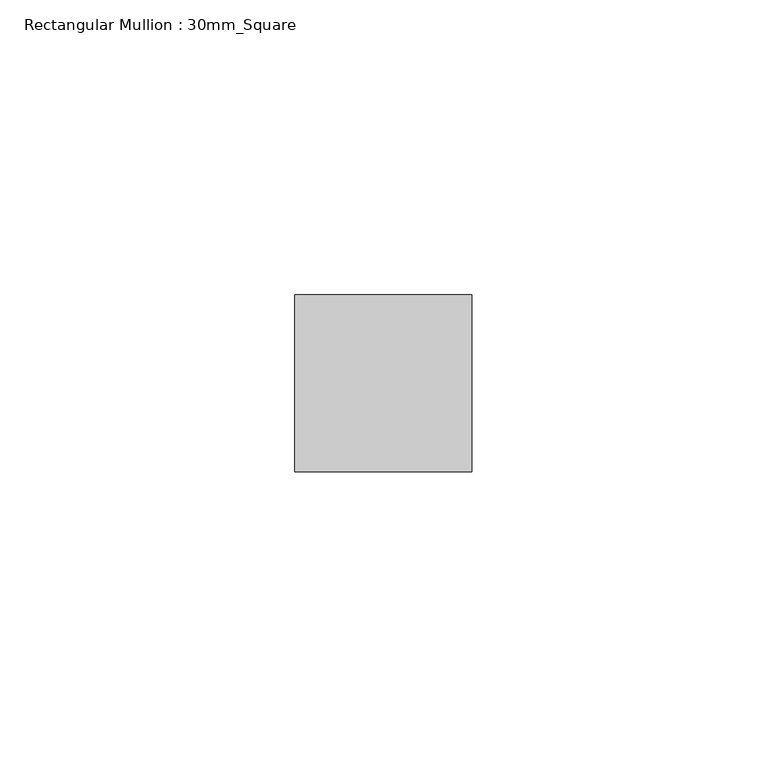
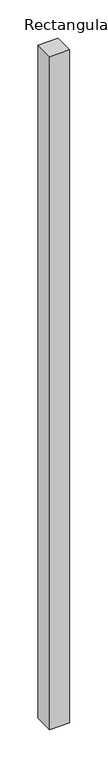
"""IFC4 building model written with IfcOpenShell, lengths in millimetres: member geometry, Rectangular Mullion : 30mm_Square."""

from ifc_helpers import new_model, si_unit, frame, origin, place, context, project, spatial, polyline, outline, extrude, source, transform, mapped, element, save


def rectangular_mullion_30mm_square_04db908b(model_context):
    return source(origin(), model_context, "Body", "SweptSolid", [
        extrude(outline(polyline([(0.0, 15.0), (0.0, -15.0), (-30.0, -15.0), (-30.0, 15.0), (0.0, 15.0)])), frame((0.0, 0.0, -1068.6296161), z_axis=(0.0, 0.0, 1.0), x_axis=(1.0, 0.0, 0.0)), (0.0, 0.0, 1.0), 1068.6296161),
    ])


if __name__ == "__main__":
    model = new_model("IFC4")
    model_context = context("Model", 3, world=origin())
    ifc_project = project(units=[si_unit("LENGTHUNIT", "METRE", prefix="MILLI")], contexts=[model_context])
    site = spatial("IfcSite", under=ifc_project)
    building = spatial("IfcBuilding", under=site)
    placement = place(None, origin())
    rectangular_mullion_30mm_square_shape = rectangular_mullion_30mm_square_04db908b(model_context)
    element("IfcMember", 1, ObjectType="Rectangular Mullion : 30mm_Square", at=placement, inside=building, context=model_context, shape_type="MappedRepresentation", body=[
        mapped(rectangular_mullion_30mm_square_shape, transform((0.0, 0.0, 0.0), x_axis=(1.0, 0.0, 0.0), y_axis=(0.0, 1.0, 0.0), z_axis=(0.0, 0.0, 1.0))),
    ])
    save(model, "model.ifc")

# Revit data of these elements
# Type "Rectangular Mullion : 30mm_Square"
#   Keynote = "H11"
#   built-in parameter 1007304 = 0.0984252 (stored number, unit not read)
#   built-in parameter 1007301 = 0.0492126 (stored number, unit not read)
#   built-in parameter 1007300 = 0.0492126 (stored number, unit not read)
# Element 1 (IfcMember, "Rectangular Mullion : 30mm_Square")
#   Materials on its faces: "Aluminium"
# Materials
#   "Aluminium": class "Metal", colour RGB 247 247 247, transparency 0, Description = "Aluminium 6061", Cost = 0
